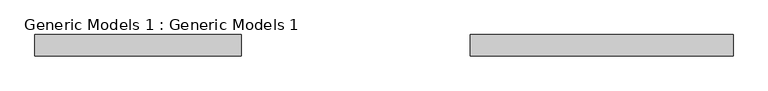
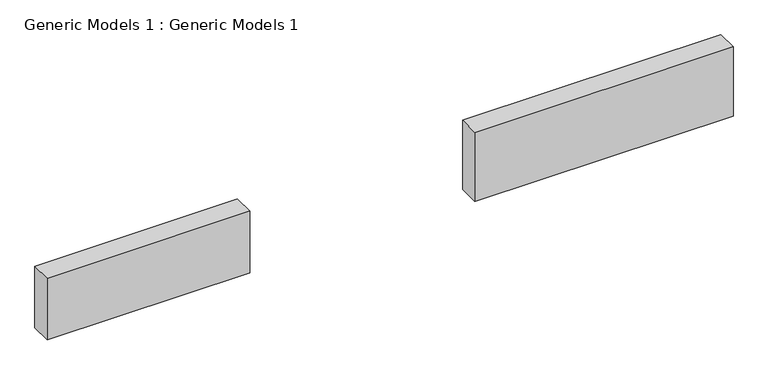
"""IFC4 building model written with IfcOpenShell, lengths in millimetres: proxy geometry, Generic Models 1 : Generic Models 1."""

from ifc_helpers import new_model, si_unit, frame, origin, place, context, project, spatial, polyline, outline, extrude, source, transform, mapped, element, save


def generic_models_1_generic_models_1_64d4bc32(model_context):
    return source(origin(), model_context, "Body", "SweptSolid", [
        extrude(outline(polyline([(4074.0046213, -9064.8675636), (314.8046213, -9064.8675636), (314.8046213, -8760.0675636), (4074.0046213, -8760.0675636), (4074.0046213, -9064.8675636)])), frame((0.0, 0.0, 289.0727456), z_axis=(0.0, 0.0, 1.0), x_axis=(1.0, 0.0, 0.0)), (0.0, 0.0, 1.0), 1065.7632544),
        extrude(outline(polyline([(-2958.7199167, -9064.8675636), (-5905.1199167, -9064.8675636), (-5905.1199167, -8760.0675636), (-2958.7199167, -8760.0675636), (-2958.7199167, -9064.8675636)])), frame((0.0, 0.0, 338.709), z_axis=(0.0, 0.0, 1.0), x_axis=(1.0, 0.0, 0.0)), (0.0, 0.0, 1.0), 948.3852),
    ])


if __name__ == "__main__":
    model = new_model("IFC4")
    model_context = context("Model", 3, world=origin())
    ifc_project = project(units=[si_unit("LENGTHUNIT", "METRE", prefix="MILLI")], contexts=[model_context])
    site = spatial("IfcSite", under=ifc_project)
    building = spatial("IfcBuilding", under=site)
    placement = place(None, origin())
    generic_models_1_generic_models_1_shape = generic_models_1_generic_models_1_64d4bc32(model_context)
    element("IfcBuildingElementProxy", 1, Name="Generic Models 1 : Generic Models 1", ObjectType="Generic Models 1 : Generic Models 1", at=placement, inside=building, context=model_context, shape_type="MappedRepresentation", body=[
        mapped(generic_models_1_generic_models_1_shape, transform((0.0, 0.0, 0.0), x_axis=(1.0, 0.0, 0.0), y_axis=(0.0, 1.0, 0.0), z_axis=(0.0, 0.0, 1.0))),
    ])
    save(model, "model.ifc")

# Revit data of these elements
# Element 1 (IfcBuildingElementProxy, "Generic Models 1 : Generic Models 1")
#   Materials on its faces: "Parking Stripe"
# Materials
#   "Parking Stripe": class "Paint", colour RGB 250 250 91, transparency 0, Cost = 0
